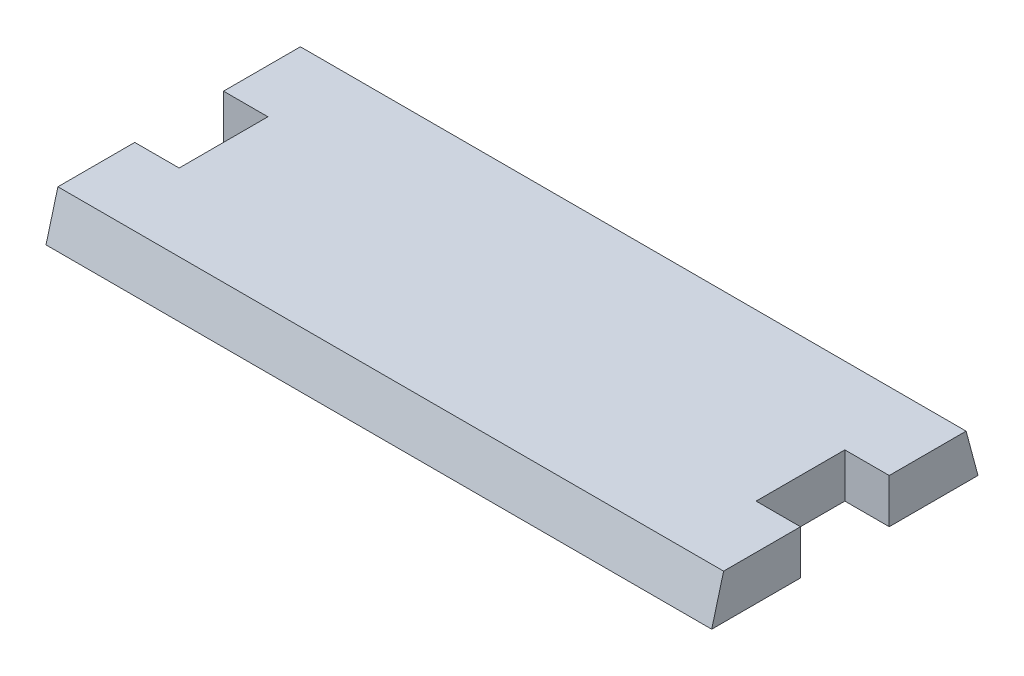
SolidWorks part; units mm, degrees
material "Plain Carbon Steel"
ref_plane "Front Plane" through (0, 0, 0) normal (0, 0, 1) x (1, 0, 0)
ref_plane "Top Plane" through (0, 0, 0) normal (0, 1, 0) x (1, 0, 0)
ref_plane "Right Plane" through (0, 0, 0) normal (1, 0, 0) x (0, 0, -1)
sketch "Top Plate Profile" plane through (0, 0, 0) normal (0, 1, 0) x (1, 0, 0)
  line L0 (-9.3913, 30) -> (177.1826, 30) construction
  line L1 (0, 0) -> (150, 0)
  line L2 (0, 0) -> (0, 20)
  line L3 (0, 60) -> (150, 60)
  line L4 (150, 0) -> (150, 20)
  line L5 (150, 40) -> (140, 40)
  line L6 (140, 40) -> (140, 20)
  line L7 (140, 20) -> (150, 20)
  line L8 (150, 40) -> (150, 60)
  line L9 (75, 0) -> (75, 43.185) construction
  line L10 (0, 40) -> (10, 40)
  line L11 (10, 40) -> (10, 20)
  line L12 (10, 20) -> (0, 20)
  line L13 (0, 40) -> (0, 60)
  dimension "D1" = 150
  dimension "D2" = 60
  dimension "D3" = 20
  dimension "D4" = 20
  dimension "D5" = 10
  dimension "D6" = 43.185
  dimension "D7" = 30
extrude "Top Plate 150x60x10" add sketch "Top Plate Profile" along normal mid plane 10
draft "Face Draft 15° A" type of draft neutral plane draft angle 15 faces to draft 1 face at (75, 0, 0) neutral plane through (0, -5, 0) neutral plane normal (0, -1, 0) reverse direction yes parameters "D1"=15
draft "Face Draft 15° B" type of draft neutral plane draft angle 15 faces to draft 1 face at (75, 0, -60) neutral plane through (0, -5, 0) neutral plane normal (0, -1, 0) reverse direction yes parameters "D1"=15
